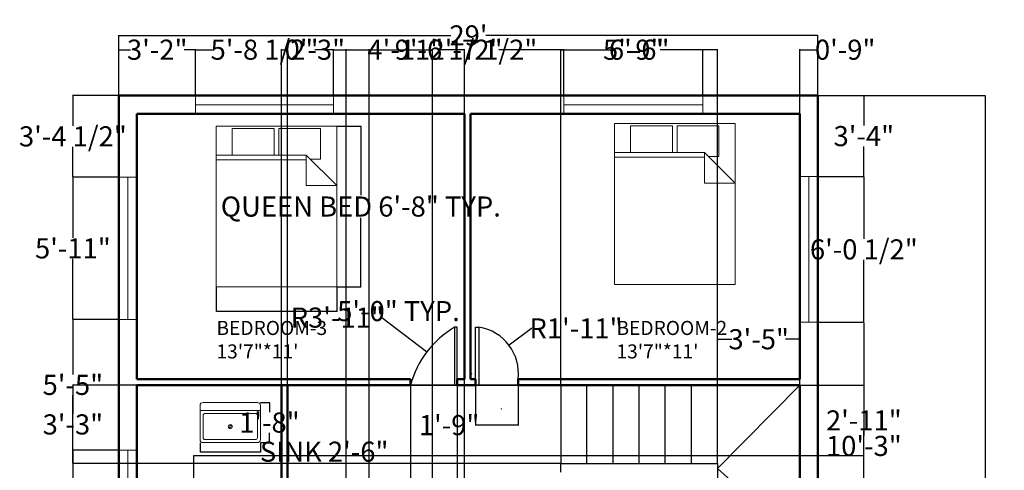
# Model space of a CAD drawing. Units: inches. Extents: x 430 to 924, y 262 to 758.
# Tile 3 of 3: x 434 to 924, y 534 to 758. Entities that reach past the tile are written whole.
import ezdxf

# ---------------------------------------------------------------- set-up
doc = ezdxf.new("R2010")
doc.units = ezdxf.units.IN
doc.header["$MEASUREMENT"] = 0
for name, color, linetype, lineweight in [('A-ANNO-DIMS', 2, 'Continuous', 18), ('A-AREA-IDEN', 7, 'Continuous', 25), ('A-DOOR', 4, 'Continuous', 25), ('A-FLOR-CASE', 9, 'Continuous', 25), ('A-FLOR-FIXT', 9, 'Continuous', 18), ('A-FLOR-STRS', 7, 'Continuous', 25), ('A-FURN', 9, 'Continuous', 18), ('A-GLAZ', 3, 'Continuous', 18), ('A-WALL', 7, 'Continuous', 50)]:
    doc.layers.add(name, color=color, linetype=linetype, lineweight=lineweight)
doc.styles.get("Standard").update_dxf_attribs({"font": 'arial.ttf'})
doc.dimstyles.get("Standard").update_dxf_attribs({"dimtxt": 10, "dimasz": 0.18, "dimexe": 0.18, "dimexo": 0.0625, "dimgap": 0.09, "dimtad": 0, "dimtih": 1, "dimtoh": 1, "dimdec": 0, "dimzin": 0, "dimdsep": 46, "dimlunit": 3, "dimtxsty": 'Standard', "dimcen": 0.09, "dimadec": 0, "dimazin": 0, "dimtfac": 1, "dimtdec": 0, "dimtofl": 0, "dimtmove": 0, "dimatfit": 3, "dimfxl": 1, "dimtolj": 1, "dimtzin": 0, "dimarcsym": 0})

# ---------------------------------------------------------------- blocks, each defined once
blk = doc.blocks.new('Bed - Queen')
for p, q in [((0, -80.00003), (0, 0)), ((0, 0), (59.99999, 0)), ((59.99999, 0), (59.99999, -80.00003)), ((7.99999, -1.2), (28.79998, -1.2)), ((7.99999, -14.4), (7.99999, -1.2)), ((28.79998, -1.2), (28.79998, -14.4)), ((31.19999, -1.2), (51.99999, -1.2)), ((31.19999, -14.4), (31.19999, -1.2)), ((51.99999, -1.2), (51.99999, -16.4)), ((0, -14.4), (44.8, -14.4)), ((59.99999, -29.6), (44.8, -14.4)), ((44.8, -14.4), (44.8, -29.6)), ((44.8, -16.8), (0, -16.8)), ((51.99999, -16.4), (46.79936, -16.4)), ((44.8, -29.6), (59.99999, -29.6)), ((59.99999, -80.00003), (0, -80.00003))]:
    blk.add_line(p, q)
blk = doc.blocks.new('Sink-single - 30 in top')
blk.add_line((-15, -3.999996), (15, -3.999996))
for points in [[(-13.5, 0), (13.5, 0)], [(-15, -18.499996), (-15, -1.5)], [(15, -1.5), (15, -18.499996)], [(-13.5, -17.499996), (-13.5, -6.499996)], [(-12.5, -5.499996), (12.5, -5.499996)], [(13.5, -6.499996), (13.5, -17.499996)], [(12.5, -18.499996), (-12.5, -18.499996)], [(13.5, -19.999996), (-13.5, -19.999996)]]:
    blk.add_lwpolyline(points)
for radius in [1, 0.5]:
    blk.add_circle((0, -11.999996), radius)
for centre, radius, start, end in [((-13.5, -1.5), 1.5, 90, 180), ((13.5, -1.5), 1.5, 0, 90), ((-12.5, -6.499996), 1, 90, 180), ((12.5, -6.499996), 1, 0, 90), ((-13.5, -18.499996), 1.5, 180, 270), ((-12.5, -17.499996), 1, 180, 270), ((12.5, -17.499996), 1, 270, 0), ((13.5, -18.499996), 1.5, 270, 0)]:
    blk.add_arc(centre, radius, start, end)
blk = doc.blocks.new('*D5')
at = {"layer": 'A-ANNO-DIMS', "color": 0, "lineweight": -2, "transparency": 16777216}
for p, q in [((483.32, 720.12), (483.32, 750.18)), ((483.5, 750), (648.65, 750)), ((831.14, 750), (665.98, 750)), ((831.32, 720.12), (831.32, 750.18))]:
    blk.add_line(p, q, dxfattribs=at)
at = {"layer": 'A-ANNO-DIMS', "color": 0, "transparency": 16777216}
for points in [[(483.5, 750.03), (483.5, 749.97), (483.32, 750)], [(831.14, 750.03), (831.14, 749.97), (831.32, 750)]]:
    blk.add_solid(points, dxfattribs=at)
at = {"layer": 'Defpoints', "color": 0, "transparency": 16777216}
for p in [(831.32, 750), (483.32, 720.05), (831.32, 720.05)]:
    blk.add_point(p, dxfattribs=at)
at = {"layer": 'A-ANNO-DIMS', "color": 0, "transparency": 16777216, "insert": (657.32, 750), "char_height": 10, "attachment_point": 5}
blk.add_mtext("\\A1;29'", dxfattribs=at)
blk = doc.blocks.new('*D6')
at = {"layer": 'A-ANNO-DIMS', "color": 0, "lineweight": -2, "transparency": 16777216}
for p, q in [((831.38, 720.05), (914.81, 720.05)), ((914.63, 719.87), (914.63, 515.25)), ((914.63, 300.23), (914.63, 504.86)), ((831.38, 300.05), (914.81, 300.05))]:
    blk.add_line(p, q, dxfattribs=at)
at = {"layer": 'A-ANNO-DIMS', "color": 0, "transparency": 16777216}
for points in [[(914.6, 719.87), (914.66, 719.87), (914.63, 720.05)], [(914.6, 300.23), (914.66, 300.23), (914.63, 300.05)]]:
    blk.add_solid(points, dxfattribs=at)
at = {"layer": 'Defpoints', "color": 0, "transparency": 16777216}
for p in [(831.32, 720.05), (831.32, 300.05), (914.63, 300.05)]:
    blk.add_point(p, dxfattribs=at)
at = {"layer": 'A-ANNO-DIMS', "color": 0, "transparency": 16777216, "insert": (914.63, 510.05), "char_height": 10, "attachment_point": 5}
blk.add_mtext("\\A1;35'", dxfattribs=at)
blk = doc.blocks.new('*D7')
at = {"layer": 'A-ANNO-DIMS', "color": 0, "lineweight": -2, "transparency": 16777216}
for p, q in [((591.83, 704.91), (603.95, 704.91)), ((603.77, 704.73), (603.77, 670.48)), ((603.77, 625.09), (603.77, 659.35)), ((591.83, 624.91), (603.95, 624.91))]:
    blk.add_line(p, q, dxfattribs=at)
at = {"layer": 'A-ANNO-DIMS', "color": 0, "transparency": 16777216}
for points in [[(603.74, 704.73), (603.8, 704.73), (603.77, 704.91)], [(603.74, 625.09), (603.8, 625.09), (603.77, 624.91)]]:
    blk.add_solid(points, dxfattribs=at)
at = {"layer": 'Defpoints', "color": 0, "transparency": 16777216}
for p in [(591.77, 704.91), (603.77, 704.91), (591.77, 624.91)]:
    blk.add_point(p, dxfattribs=at)
at = {"layer": 'A-ANNO-DIMS', "color": 0, "transparency": 16777216, "insert": (603.77, 664.91), "char_height": 10, "attachment_point": 5}
blk.add_mtext('\\A1;QUEEN BED 6\'-8" TYP.', dxfattribs=at)
blk = doc.blocks.new('*D8')
at = {"layer": 'A-ANNO-DIMS', "color": 0, "lineweight": -2, "transparency": 16777216}
for p, q in [((531.77, 624.85), (531.77, 612.73)), ((591.77, 624.85), (591.77, 612.73)), ((531.95, 612.91), (591.59, 612.91)), ((591.77, 612.91), (591.95, 612.91))]:
    blk.add_line(p, q, dxfattribs=at)
at = {"layer": 'A-ANNO-DIMS', "color": 0, "transparency": 16777216}
for points in [[(531.95, 612.94), (531.95, 612.88), (531.77, 612.91)], [(591.59, 612.94), (591.59, 612.88), (591.77, 612.91)]]:
    blk.add_solid(points, dxfattribs=at)
at = {"layer": 'Defpoints', "color": 0, "transparency": 16777216}
for p in [(531.77, 624.91), (591.77, 624.91), (591.77, 612.91)]:
    blk.add_point(p, dxfattribs=at)
at = {"layer": 'A-ANNO-DIMS', "color": 0, "transparency": 16777216, "insert": (622.52, 612.91), "char_height": 10, "attachment_point": 5}
blk.add_mtext('\\A1;5\'-0" TYP.', dxfattribs=at)
blk = doc.blocks.new('*D11')
at = {"layer": 'A-ANNO-DIMS', "color": 0, "lineweight": -2, "transparency": 16777216}
for p, q in [((523.75, 547.42), (523.75, 542.8)), ((553.75, 547.42), (553.75, 542.8)), ((523.93, 542.98), (553.57, 542.98)), ((553.75, 542.98), (553.93, 542.98))]:
    blk.add_line(p, q, dxfattribs=at)
at = {"layer": 'A-ANNO-DIMS', "color": 0, "transparency": 16777216}
for points in [[(523.93, 543.01), (523.93, 542.95), (523.75, 542.98)], [(553.57, 543.01), (553.57, 542.95), (553.75, 542.98)]]:
    blk.add_solid(points, dxfattribs=at)
at = {"layer": 'Defpoints', "color": 0, "transparency": 16777216}
for p in [(523.75, 547.48), (553.75, 547.48), (553.75, 542.98)]:
    blk.add_point(p, dxfattribs=at)
at = {"layer": 'A-ANNO-DIMS', "color": 0, "transparency": 16777216, "insert": (585.53, 542.98), "char_height": 10, "attachment_point": 5}
blk.add_mtext('\\A1;SINK 2\'-6"', dxfattribs=at)
blk = doc.blocks.new('*D12')
at = {"layer": 'A-ANNO-DIMS', "color": 0, "lineweight": -2, "transparency": 16777216}
for p, q in [((553.82, 567.48), (558.43, 567.48)), ((558.25, 567.3), (558.25, 562.68)), ((558.25, 547.66), (558.25, 552.29)), ((553.82, 547.48), (558.43, 547.48))]:
    blk.add_line(p, q, dxfattribs=at)
at = {"layer": 'A-ANNO-DIMS', "color": 0, "transparency": 16777216}
for points in [[(558.22, 567.3), (558.28, 567.3), (558.25, 567.48)], [(558.22, 547.66), (558.28, 547.66), (558.25, 547.48)]]:
    blk.add_solid(points, dxfattribs=at)
at = {"layer": 'Defpoints', "color": 0, "transparency": 16777216}
for p in [(553.75, 567.48), (558.25, 567.48), (553.75, 547.48)]:
    blk.add_point(p, dxfattribs=at)
at = {"layer": 'A-ANNO-DIMS', "color": 0, "transparency": 16777216, "insert": (558.25, 557.48), "char_height": 10, "attachment_point": 5}
blk.add_mtext('\\A1;1\'-8"', dxfattribs=at)
blk = doc.blocks.new('*D15')
at = {"layer": 'A-ANNO-DIMS', "color": 0, "lineweight": -2, "transparency": 16777216}
for p, q in [((483.32, 720.12), (483.32, 743.09)), ((483.5, 742.91), (489.04, 742.91)), ((521.35, 742.91), (515.8, 742.91)), ((521.53, 720.12), (521.53, 743.09))]:
    blk.add_line(p, q, dxfattribs=at)
at = {"layer": 'A-ANNO-DIMS', "color": 0, "transparency": 16777216}
for points in [[(483.5, 742.94), (483.5, 742.88), (483.32, 742.91)], [(521.35, 742.94), (521.35, 742.88), (521.53, 742.91)]]:
    blk.add_solid(points, dxfattribs=at)
at = {"layer": 'Defpoints', "color": 0, "transparency": 16777216}
for p in [(521.53, 742.91), (483.32, 720.05), (521.53, 720.05)]:
    blk.add_point(p, dxfattribs=at)
at = {"layer": 'A-ANNO-DIMS', "color": 0, "transparency": 16777216, "insert": (502.42, 742.91), "char_height": 10, "attachment_point": 5}
blk.add_mtext('\\A1;3\'-2"', dxfattribs=at)
blk = doc.blocks.new('*D16')
at = {"layer": 'A-ANNO-DIMS', "color": 0, "lineweight": -2, "transparency": 16777216}
for p, q in [((521.53, 720.12), (521.53, 743.09)), ((521.71, 742.91), (530.79, 742.91)), ((589.94, 742.91), (580.86, 742.91)), ((590.12, 720.12), (590.12, 743.09))]:
    blk.add_line(p, q, dxfattribs=at)
at = {"layer": 'A-ANNO-DIMS', "color": 0, "transparency": 16777216}
for points in [[(521.71, 742.94), (521.71, 742.88), (521.53, 742.91)], [(589.94, 742.94), (589.94, 742.88), (590.12, 742.91)]]:
    blk.add_solid(points, dxfattribs=at)
at = {"layer": 'Defpoints', "color": 0, "transparency": 16777216}
for p in [(590.12, 742.91), (521.53, 720.05), (590.12, 720.05)]:
    blk.add_point(p, dxfattribs=at)
at = {"layer": 'A-ANNO-DIMS', "color": 0, "transparency": 16777216, "insert": (555.83, 742.91), "char_height": 10, "attachment_point": 5}
blk.add_mtext('\\A1;5\'-8 1/2"', dxfattribs=at)
blk = doc.blocks.new('*D17')
at = {"layer": 'A-ANNO-DIMS', "color": 0, "lineweight": -2, "transparency": 16777216}
for p, q in [((590.12, 720.12), (590.12, 743.09)), ((590.3, 742.91), (622.43, 742.91)), ((704.63, 742.91), (672.5, 742.91)), ((704.81, 720.12), (704.81, 743.09))]:
    blk.add_line(p, q, dxfattribs=at)
at = {"layer": 'A-ANNO-DIMS', "color": 0, "transparency": 16777216}
for points in [[(590.3, 742.94), (590.3, 742.88), (590.12, 742.91)], [(704.63, 742.94), (704.63, 742.88), (704.81, 742.91)]]:
    blk.add_solid(points, dxfattribs=at)
at = {"layer": 'Defpoints', "color": 0, "transparency": 16777216}
for p in [(704.81, 742.91), (590.12, 720.05), (704.81, 720.05)]:
    blk.add_point(p, dxfattribs=at)
at = {"layer": 'A-ANNO-DIMS', "color": 0, "transparency": 16777216, "insert": (647.47, 742.91), "char_height": 10, "attachment_point": 5}
blk.add_mtext('\\A1;9\'-6 1/2"', dxfattribs=at)
blk = doc.blocks.new('*D18')
at = {"layer": 'A-ANNO-DIMS', "color": 0, "lineweight": -2, "transparency": 16777216}
for p, q in [((704.81, 720.12), (704.81, 743.09)), ((704.99, 742.91), (726, 742.91)), ((773.78, 742.91), (752.76, 742.91)), ((773.96, 720.12), (773.96, 743.09))]:
    blk.add_line(p, q, dxfattribs=at)
at = {"layer": 'A-ANNO-DIMS', "color": 0, "transparency": 16777216}
for points in [[(704.99, 742.94), (704.99, 742.88), (704.81, 742.91)], [(773.78, 742.94), (773.78, 742.88), (773.96, 742.91)]]:
    blk.add_solid(points, dxfattribs=at)
at = {"layer": 'Defpoints', "color": 0, "transparency": 16777216}
for p in [(773.96, 742.91), (704.81, 720.05), (773.96, 720.05)]:
    blk.add_point(p, dxfattribs=at)
at = {"layer": 'A-ANNO-DIMS', "color": 0, "transparency": 16777216, "insert": (739.38, 742.91), "char_height": 10, "attachment_point": 5}
blk.add_mtext('\\A1;5\'-9"', dxfattribs=at)
blk = doc.blocks.new('*D19')
at = {"layer": 'A-ANNO-DIMS', "color": 0, "lineweight": -2, "transparency": 16777216}
for p, q in [((831.38, 720.05), (854.35, 720.05)), ((854.17, 719.87), (854.17, 705.14)), ((854.17, 680.01), (854.17, 694.75)), ((831.38, 679.83), (854.35, 679.83))]:
    blk.add_line(p, q, dxfattribs=at)
at = {"layer": 'A-ANNO-DIMS', "color": 0, "transparency": 16777216}
for points in [[(854.14, 719.87), (854.2, 719.87), (854.17, 720.05)], [(854.14, 680.01), (854.2, 680.01), (854.17, 679.83)]]:
    blk.add_solid(points, dxfattribs=at)
at = {"layer": 'Defpoints', "color": 0, "transparency": 16777216}
for p in [(831.32, 720.05), (831.32, 679.83), (854.17, 679.83)]:
    blk.add_point(p, dxfattribs=at)
at = {"layer": 'A-ANNO-DIMS', "color": 0, "transparency": 16777216, "insert": (854.17, 699.94), "char_height": 10, "attachment_point": 5}
blk.add_mtext('\\A1;3\'-4"', dxfattribs=at)
blk = doc.blocks.new('*D20')
at = {"layer": 'A-ANNO-DIMS', "color": 0, "lineweight": -2, "transparency": 16777216}
for p, q in [((831.38, 679.83), (854.35, 679.83)), ((854.17, 679.65), (854.17, 648.84)), ((854.17, 607.5), (854.17, 638.32)), ((831.38, 607.32), (854.35, 607.32))]:
    blk.add_line(p, q, dxfattribs=at)
at = {"layer": 'A-ANNO-DIMS', "color": 0, "transparency": 16777216}
for points in [[(854.14, 679.65), (854.2, 679.65), (854.17, 679.83)], [(854.14, 607.5), (854.2, 607.5), (854.17, 607.32)]]:
    blk.add_solid(points, dxfattribs=at)
at = {"layer": 'Defpoints', "color": 0, "transparency": 16777216}
for p in [(831.32, 679.83), (831.32, 607.32), (854.17, 607.32)]:
    blk.add_point(p, dxfattribs=at)
at = {"layer": 'A-ANNO-DIMS', "color": 0, "transparency": 16777216, "insert": (854.17, 643.58), "char_height": 10, "attachment_point": 5}
blk.add_mtext('\\A1;6\'-0 1/2"', dxfattribs=at)
blk = doc.blocks.new('*D21')
at = {"layer": 'A-ANNO-DIMS', "color": 0, "lineweight": -2, "transparency": 16777216}
for p, q in [((831.38, 607.32), (854.35, 607.32)), ((854.17, 607.14), (854.17, 551.05)), ((854.17, 484.56), (854.17, 540.65)), ((831.38, 484.38), (854.35, 484.38))]:
    blk.add_line(p, q, dxfattribs=at)
at = {"layer": 'A-ANNO-DIMS', "color": 0, "transparency": 16777216}
for points in [[(854.14, 607.14), (854.2, 607.14), (854.17, 607.32)], [(854.14, 484.56), (854.2, 484.56), (854.17, 484.38)]]:
    blk.add_solid(points, dxfattribs=at)
at = {"layer": 'Defpoints', "color": 0, "transparency": 16777216}
for p in [(831.32, 607.32), (831.32, 484.38), (854.17, 484.38)]:
    blk.add_point(p, dxfattribs=at)
at = {"layer": 'A-ANNO-DIMS', "color": 0, "transparency": 16777216, "insert": (854.17, 545.85), "char_height": 10, "attachment_point": 5}
blk.add_mtext('\\A1;10\'-3"', dxfattribs=at)
blk = doc.blocks.new('*D25')
at = {"layer": 'A-ANNO-DIMS', "color": 0, "lineweight": -2, "transparency": 16777216}
for p, q in [((483.25, 720.05), (460.24, 720.05)), ((460.42, 719.87), (460.42, 705.08)), ((460.42, 679.75), (460.42, 694.55)), ((483.25, 679.57), (460.24, 679.57))]:
    blk.add_line(p, q, dxfattribs=at)
at = {"layer": 'A-ANNO-DIMS', "color": 0, "transparency": 16777216}
for points in [[(460.39, 719.87), (460.45, 719.87), (460.42, 720.05)], [(460.39, 679.75), (460.45, 679.75), (460.42, 679.57)]]:
    blk.add_solid(points, dxfattribs=at)
at = {"layer": 'Defpoints', "color": 0, "transparency": 16777216}
for p in [(483.32, 720.05), (460.42, 679.57), (483.32, 679.57)]:
    blk.add_point(p, dxfattribs=at)
at = {"layer": 'A-ANNO-DIMS', "color": 0, "transparency": 16777216, "insert": (460.42, 699.81), "char_height": 10, "attachment_point": 5}
blk.add_mtext('\\A1;3\'-4 1/2"', dxfattribs=at)
blk = doc.blocks.new('*D26')
at = {"layer": 'A-ANNO-DIMS', "color": 0, "lineweight": -2, "transparency": 16777216}
for p, q in [((483.25, 679.57), (460.24, 679.57)), ((460.42, 679.39), (460.42, 649.31)), ((460.42, 608.84), (460.42, 638.92)), ((483.25, 608.66), (460.24, 608.66))]:
    blk.add_line(p, q, dxfattribs=at)
at = {"layer": 'A-ANNO-DIMS', "color": 0, "transparency": 16777216}
for points in [[(460.39, 679.39), (460.45, 679.39), (460.42, 679.57)], [(460.39, 608.84), (460.45, 608.84), (460.42, 608.66)]]:
    blk.add_solid(points, dxfattribs=at)
at = {"layer": 'Defpoints', "color": 0, "transparency": 16777216}
for p in [(483.32, 679.57), (460.42, 608.66), (483.32, 608.66)]:
    blk.add_point(p, dxfattribs=at)
at = {"layer": 'A-ANNO-DIMS', "color": 0, "transparency": 16777216, "insert": (460.42, 644.11), "char_height": 10, "attachment_point": 5}
blk.add_mtext('\\A1;5\'-11"', dxfattribs=at)
blk = doc.blocks.new('*D27')
at = {"layer": 'A-ANNO-DIMS', "color": 0, "lineweight": -2, "transparency": 16777216}
for p, q in [((483.25, 608.66), (460.24, 608.66)), ((460.42, 608.48), (460.42, 581.39)), ((460.42, 543.96), (460.42, 571.04)), ((483.25, 543.78), (460.24, 543.78))]:
    blk.add_line(p, q, dxfattribs=at)
at = {"layer": 'A-ANNO-DIMS', "color": 0, "transparency": 16777216}
for points in [[(460.39, 608.48), (460.45, 608.48), (460.42, 608.66)], [(460.39, 543.96), (460.45, 543.96), (460.42, 543.78)]]:
    blk.add_solid(points, dxfattribs=at)
at = {"layer": 'Defpoints', "color": 0, "transparency": 16777216}
for p in [(483.32, 608.66), (460.42, 543.78), (483.32, 543.78)]:
    blk.add_point(p, dxfattribs=at)
at = {"layer": 'A-ANNO-DIMS', "color": 0, "transparency": 16777216, "insert": (460.42, 576.22), "char_height": 10, "attachment_point": 5}
blk.add_mtext('\\A1;5\'-5"', dxfattribs=at)
blk = doc.blocks.new('*D28')
at = {"layer": 'A-ANNO-DIMS', "color": 0, "lineweight": -2, "transparency": 16777216}
for p, q in [((483.25, 543.78), (460.24, 543.78)), ((460.42, 543.6), (460.42, 518.31)), ((460.42, 482.49), (460.42, 507.78)), ((483.25, 482.31), (460.24, 482.31))]:
    blk.add_line(p, q, dxfattribs=at)
at = {"layer": 'A-ANNO-DIMS', "color": 0, "transparency": 16777216}
for points in [[(460.39, 543.6), (460.45, 543.6), (460.42, 543.78)], [(460.39, 482.49), (460.45, 482.49), (460.42, 482.31)]]:
    blk.add_solid(points, dxfattribs=at)
at = {"layer": 'Defpoints', "color": 0, "transparency": 16777216}
for p in [(483.32, 543.78), (460.42, 482.31), (483.32, 482.31)]:
    blk.add_point(p, dxfattribs=at)
at = {"layer": 'A-ANNO-DIMS', "color": 0, "transparency": 16777216, "insert": (460.42, 513.05), "char_height": 10, "attachment_point": 5}
blk.add_mtext('\\A1;5\'-1 1/2"', dxfattribs=at)
blk = doc.blocks.new('*D35')
at = {"layer": 'A-ANNO-DIMS', "color": 0, "lineweight": -2, "transparency": 16777216}
for p, q in [((596.53, 380.21), (596.53, 743.09)), ((596.71, 742.91), (608.45, 742.91)), ((655.14, 742.91), (643.39, 742.91)), ((655.32, 380.21), (655.32, 743.09))]:
    blk.add_line(p, q, dxfattribs=at)
at = {"layer": 'A-ANNO-DIMS', "color": 0, "transparency": 16777216}
for points in [[(596.71, 742.94), (596.71, 742.88), (596.53, 742.91)], [(655.14, 742.94), (655.14, 742.88), (655.32, 742.91)]]:
    blk.add_solid(points, dxfattribs=at)
at = {"layer": 'Defpoints', "color": 0, "transparency": 16777216}
for p in [(655.32, 742.91), (596.53, 380.15), (655.32, 380.15)]:
    blk.add_point(p, dxfattribs=at)
at = {"layer": 'A-ANNO-DIMS', "color": 0, "transparency": 16777216, "insert": (625.92, 742.91), "char_height": 10, "attachment_point": 5}
blk.add_mtext('\\A1;4\'-11"', dxfattribs=at)
blk = doc.blocks.new('*D36')
at = {"layer": 'A-ANNO-DIMS', "color": 0, "lineweight": -2, "transparency": 16777216}
for p, q in [((703.32, 576.12), (703.32, 743.09)), ((703.5, 742.91), (728.92, 742.91)), ((781.17, 742.91), (755.74, 742.91)), ((781.35, 576.12), (781.35, 743.09))]:
    blk.add_line(p, q, dxfattribs=at)
at = {"layer": 'A-ANNO-DIMS', "color": 0, "transparency": 16777216}
for points in [[(703.5, 742.94), (703.5, 742.88), (703.32, 742.91)], [(781.17, 742.94), (781.17, 742.88), (781.35, 742.91)]]:
    blk.add_solid(points, dxfattribs=at)
at = {"layer": 'Defpoints', "color": 0, "transparency": 16777216}
for p in [(781.35, 742.91), (703.32, 576.05), (781.35, 576.05)]:
    blk.add_point(p, dxfattribs=at)
at = {"layer": 'A-ANNO-DIMS', "color": 0, "transparency": 16777216, "insert": (742.33, 742.91), "char_height": 10, "attachment_point": 5}
blk.add_mtext('\\A1;6\'-6"', dxfattribs=at)
blk = doc.blocks.new('*D37')
at = {"layer": 'A-ANNO-DIMS', "color": 0, "lineweight": -2, "transparency": 16777216}
for p, q in [((781.35, 576.12), (781.35, 599.09)), ((781.53, 598.91), (788.45, 598.91)), ((822.14, 598.91), (815.21, 598.91)), ((822.32, 576.12), (822.32, 599.09))]:
    blk.add_line(p, q, dxfattribs=at)
at = {"layer": 'A-ANNO-DIMS', "color": 0, "transparency": 16777216}
for points in [[(781.53, 598.94), (781.53, 598.88), (781.35, 598.91)], [(822.14, 598.94), (822.14, 598.88), (822.32, 598.91)]]:
    blk.add_solid(points, dxfattribs=at)
at = {"layer": 'Defpoints', "color": 0, "transparency": 16777216}
for p in [(822.32, 598.91), (781.35, 576.05), (822.32, 576.05)]:
    blk.add_point(p, dxfattribs=at)
at = {"layer": 'A-ANNO-DIMS', "color": 0, "transparency": 16777216, "insert": (801.83, 598.91), "char_height": 10, "attachment_point": 5}
blk.add_mtext('\\A1;3\'-5"', dxfattribs=at)
blk = doc.blocks.new('*D38')
at = {"layer": 'A-ANNO-DIMS', "color": 0, "lineweight": -2, "transparency": 16777216}
for p, q in [((703.25, 576.05), (460.24, 576.05)), ((460.42, 575.87), (460.42, 561.75)), ((460.42, 537.23), (460.42, 551.36)), ((703.25, 537.05), (460.24, 537.05))]:
    blk.add_line(p, q, dxfattribs=at)
at = {"layer": 'A-ANNO-DIMS', "color": 0, "transparency": 16777216}
for points in [[(460.39, 575.87), (460.45, 575.87), (460.42, 576.05)], [(460.39, 537.23), (460.45, 537.23), (460.42, 537.05)]]:
    blk.add_solid(points, dxfattribs=at)
at = {"layer": 'Defpoints', "color": 0, "transparency": 16777216}
for p in [(703.32, 576.05), (460.42, 537.05), (703.32, 537.05)]:
    blk.add_point(p, dxfattribs=at)
at = {"layer": 'A-ANNO-DIMS', "color": 0, "transparency": 16777216, "insert": (460.42, 556.55), "char_height": 10, "attachment_point": 5}
blk.add_mtext('\\A1;3\'-3"', dxfattribs=at)
blk = doc.blocks.new('*D41')
at = {"layer": 'A-ANNO-DIMS', "color": 0, "lineweight": -2, "transparency": 16777216}
for p, q in [((822.32, 484.44), (822.32, 743.09)), ((822.5, 742.91), (831.14, 742.91)), ((831.32, 484.44), (831.32, 743.09)), ((831.32, 742.91), (831.5, 742.91))]:
    blk.add_line(p, q, dxfattribs=at)
at = {"layer": 'A-ANNO-DIMS', "color": 0, "transparency": 16777216}
for points in [[(822.5, 742.94), (822.5, 742.88), (822.32, 742.91)], [(831.14, 742.94), (831.14, 742.88), (831.32, 742.91)]]:
    blk.add_solid(points, dxfattribs=at)
at = {"layer": 'Defpoints', "color": 0, "transparency": 16777216}
for p in [(831.32, 742.91), (822.32, 484.38), (831.32, 484.38)]:
    blk.add_point(p, dxfattribs=at)
at = {"layer": 'A-ANNO-DIMS', "color": 0, "transparency": 16777216, "insert": (844.88, 742.91), "char_height": 10, "attachment_point": 5}
blk.add_mtext('\\A1;0\'-9"', dxfattribs=at)
blk = doc.blocks.new('*D43')
at = {"layer": 'A-ANNO-DIMS', "color": 0, "lineweight": -2, "transparency": 16777216}
for p, q in [((564.38, 576.05), (854.35, 576.05)), ((854.17, 575.87), (854.17, 563.64)), ((854.17, 541.19), (854.17, 553.42)), ((564.38, 541.01), (854.35, 541.01))]:
    blk.add_line(p, q, dxfattribs=at)
at = {"layer": 'A-ANNO-DIMS', "color": 0, "transparency": 16777216}
for points in [[(854.14, 575.87), (854.2, 575.87), (854.17, 576.05)], [(854.14, 541.19), (854.2, 541.19), (854.17, 541.01)]]:
    blk.add_solid(points, dxfattribs=at)
at = {"layer": 'Defpoints', "color": 0, "transparency": 16777216}
for p in [(564.32, 576.05), (854.17, 576.05), (564.32, 541.01)]:
    blk.add_point(p, dxfattribs=at)
at = {"layer": 'A-ANNO-DIMS', "color": 0, "transparency": 16777216, "insert": (854.17, 558.53), "char_height": 10, "attachment_point": 5}
blk.add_mtext('\\A1;2\'-11"', dxfattribs=at)
blk = doc.blocks.new('*D45')
at = {"layer": 'A-ANNO-DIMS', "color": 0, "lineweight": -2, "transparency": 16777216}
for p, q in [((564.32, 576.12), (564.32, 743.09)), ((564.5, 742.91), (567.14, 742.91)), ((567.32, 576.12), (567.32, 743.09)), ((567.32, 742.91), (567.5, 742.91))]:
    blk.add_line(p, q, dxfattribs=at)
at = {"layer": 'A-ANNO-DIMS', "color": 0, "transparency": 16777216}
for points in [[(564.5, 742.94), (564.5, 742.88), (564.32, 742.91)], [(567.14, 742.94), (567.14, 742.88), (567.32, 742.91)]]:
    blk.add_solid(points, dxfattribs=at)
at = {"layer": 'Defpoints', "color": 0, "transparency": 16777216}
for p in [(567.32, 742.91), (564.32, 576.05), (567.32, 576.05)]:
    blk.add_point(p, dxfattribs=at)
at = {"layer": 'A-ANNO-DIMS', "color": 0, "transparency": 16777216, "insert": (580.88, 742.91), "char_height": 10, "attachment_point": 5}
blk.add_mtext('\\A1;0\'-3"', dxfattribs=at)
blk = doc.blocks.new('*D46')
at = {"layer": 'A-ANNO-DIMS', "color": 0, "lineweight": -2, "transparency": 16777216}
for p, q in [((628.55, 575.99), (628.55, 277.02)), ((651.7, 575.99), (651.7, 277.02)), ((628.73, 277.2), (651.52, 277.2)), ((651.7, 277.2), (651.88, 277.2))]:
    blk.add_line(p, q, dxfattribs=at)
at = {"layer": 'A-ANNO-DIMS', "color": 0, "transparency": 16777216}
for points in [[(628.73, 277.23), (628.73, 277.17), (628.55, 277.2)], [(651.52, 277.23), (651.52, 277.17), (651.7, 277.2)]]:
    blk.add_solid(points, dxfattribs=at)
at = {"layer": 'Defpoints', "color": 0, "transparency": 16777216}
for p in [(628.55, 576.05), (651.7, 576.05), (651.7, 277.2)]:
    blk.add_point(p, dxfattribs=at)
at = {"layer": 'A-ANNO-DIMS', "color": 0, "transparency": 16777216, "insert": (668.68, 277.2), "char_height": 10, "attachment_point": 5}
blk.add_mtext('\\A1;1\'-11"', dxfattribs=at)
blk = doc.blocks.new('*D47')
at = {"layer": 'A-ANNO-DIMS', "color": 0, "lineweight": -2, "transparency": 16777216}
for p, q in [((660.82, 578.99), (660.82, 556.02)), ((682.01, 578.99), (682.01, 556.02)), ((660.82, 556.2), (660.64, 556.2)), ((681.83, 556.2), (661, 556.2))]:
    blk.add_line(p, q, dxfattribs=at)
at = {"layer": 'A-ANNO-DIMS', "color": 0, "transparency": 16777216}
for points in [[(661, 556.23), (661, 556.17), (660.82, 556.2)], [(681.83, 556.23), (681.83, 556.17), (682.01, 556.2)]]:
    blk.add_solid(points, dxfattribs=at)
at = {"layer": 'Defpoints', "color": 0, "transparency": 16777216}
for p in [(660.82, 579.05), (682.01, 579.05), (660.82, 556.2)]:
    blk.add_point(p, dxfattribs=at)
at = {"layer": 'A-ANNO-DIMS', "color": 0, "transparency": 16777216, "insert": (647.73, 556.2), "char_height": 10, "attachment_point": 5}
blk.add_mtext('\\A1;1\'-9"', dxfattribs=at)
blk = doc.blocks.new('*D48')
at = {"layer": 'A-ANNO-DIMS', "color": 0, "lineweight": -2, "transparency": 16777216}
for p, q in [((607.88, 405.12), (607.88, 743.09)), ((608.06, 742.91), (639.32, 742.91)), ((639.5, 405.12), (639.5, 743.09)), ((639.5, 742.91), (639.68, 742.91))]:
    blk.add_line(p, q, dxfattribs=at)
at = {"layer": 'A-ANNO-DIMS', "color": 0, "transparency": 16777216}
for points in [[(608.06, 742.94), (608.06, 742.88), (607.88, 742.91)], [(639.32, 742.94), (639.32, 742.88), (639.5, 742.91)]]:
    blk.add_solid(points, dxfattribs=at)
at = {"layer": 'Defpoints', "color": 0, "transparency": 16777216}
for p in [(639.5, 742.91), (607.88, 405.05), (639.5, 405.05)]:
    blk.add_point(p, dxfattribs=at)
at = {"layer": 'A-ANNO-DIMS', "color": 0, "transparency": 16777216, "insert": (664.79, 742.91), "char_height": 10, "attachment_point": 5}
blk.add_mtext('\\A1;2\'-7 1/2"', dxfattribs=at)
blk = doc.blocks.new('*D52')
at = {"layer": 'A-ANNO-DIMS', "color": 0, "lineweight": -2, "transparency": 16777216}
for p, q in [((614.09, 609.68), (614.27, 609.68)), ((614.27, 609.68), (636.47, 592.79)), ((673.76, 564.35), (673.94, 564.35)), ((673.85, 564.26), (673.85, 564.44))]:
    blk.add_line(p, q, dxfattribs=at)
at = {"layer": 'A-ANNO-DIMS', "color": 0, "transparency": 16777216}
blk.add_solid([(636.49, 592.81), (636.45, 592.77), (636.61, 592.68)], dxfattribs=at)
at = {"layer": 'Defpoints', "color": 0, "transparency": 16777216}
for p in [(636.61, 592.68), (673.85, 564.35)]:
    blk.add_point(p, dxfattribs=at)
at = {"layer": 'A-ANNO-DIMS', "color": 0, "transparency": 16777216, "insert": (592.04, 609.68), "char_height": 10, "attachment_point": 5}
blk.add_mtext('\\A1;R3\'-11"', dxfattribs=at)
blk = doc.blocks.new('*D53')
at = {"layer": 'A-ANNO-DIMS', "color": 0, "lineweight": -2, "transparency": 16777216}
for p, q in [((688.65, 604.3), (677.66, 596.02)), ((688.83, 604.3), (688.65, 604.3)), ((658.87, 581.93), (659.05, 581.93)), ((658.96, 581.84), (658.96, 582.02))]:
    blk.add_line(p, q, dxfattribs=at)
at = {"layer": 'A-ANNO-DIMS', "color": 0, "transparency": 16777216}
blk.add_solid([(677.64, 596.04), (677.68, 596), (677.52, 595.91)], dxfattribs=at)
at = {"layer": 'Defpoints', "color": 0, "transparency": 16777216}
for p in [(677.52, 595.91), (658.96, 581.93)]:
    blk.add_point(p, dxfattribs=at)
at = {"layer": 'A-ANNO-DIMS', "color": 0, "transparency": 16777216, "insert": (710.89, 604.3), "char_height": 10, "attachment_point": 5}
blk.add_mtext('\\A1;R1\'-11"', dxfattribs=at)

msp = doc.modelspace()

# ---------------------------------------------------------------- linework, layer by layer
at = {"layer": 'A-DOOR'}
for p, q in [((651.7, 604.89), (650.48, 604.89)), ((650.48, 604.89), (650.48, 576.05)), ((651.7, 579.05), (651.7, 604.89)), ((660.82, 579.05), (660.82, 604.89)), ((660.82, 604.89), (662.56, 604.89)), ((662.56, 604.89), (662.56, 576.05)), ((628.55, 576.05), (648.07, 576.05)), ((651.7, 576.05), (648.07, 576.05)), ((660.82, 576.05), (663.66, 576.05)), ((682.01, 576.05), (663.66, 576.05))]:
    msp.add_line(p, q, dxfattribs=at)
for centre, radius, start, end in [((673.85, 564.35), 46.79, 119.9685, 165.5188), ((658.96, 581.93), 23.24, 352.8813, 81.0788)]:
    msp.add_arc(centre, radius, start, end, dxfattribs=at)
at = {"layer": 'A-FLOR-CASE'}
for p, q in [((520.6, 456.05), (520.6, 541.01)), ((520.6, 541.01), (564.32, 541.01))]:
    msp.add_line(p, q, dxfattribs=at)
at = {"layer": 'A-FLOR-STRS'}
for p, q in [((703.32, 576.05), (703.32, 537.05)), ((716.35, 537.05), (716.35, 576.05)), ((729.35, 537.05), (729.35, 576.05)), ((742.35, 537.05), (742.35, 576.05)), ((755.35, 537.05), (755.35, 576.05)), ((768.35, 537.05), (768.35, 576.05)), ((781.35, 537.05), (781.35, 576.05)), ((781.35, 534.67), (822.32, 576.05)), ((703.32, 537.05), (781.16, 537.05)), ((703.32, 532.81), (703.32, 537.05)), ((781.35, 537.05), (781.16, 537.05)), ((781.35, 537.05), (781.35, 498.05)), ((781.35, 534.67), (822.32, 498.05))]:
    msp.add_line(p, q, dxfattribs=at)
at = {"layer": 'A-GLAZ'}
for p, q in [((521.53, 720.05), (521.53, 711.05)), ((590.12, 720.05), (590.12, 711.05)), ((704.81, 711.05), (704.81, 720.05)), ((773.96, 720.05), (773.96, 711.05)), ((521.53, 715.55), (590.12, 715.55)), ((704.81, 715.55), (773.96, 715.55)), ((483.32, 679.57), (492.32, 679.57)), ((487.82, 679.57), (487.82, 608.66)), ((822.32, 679.83), (831.32, 679.83)), ((826.82, 679.83), (826.82, 607.32)), ((483.32, 608.66), (492.32, 608.66)), ((822.32, 607.32), (831.32, 607.32)), ((483.32, 543.78), (492.32, 543.78)), ((487.82, 543.78), (487.82, 482.31))]:
    msp.add_line(p, q, dxfattribs=at)
at = {"layer": 'A-WALL'}
for p, q in [((492.32, 711.05), (655.32, 711.05)), ((492.32, 579.05), (492.32, 711.05)), ((655.32, 579.05), (655.32, 711.05)), ((658.32, 579.05), (658.32, 711.05)), ((658.32, 711.05), (822.32, 711.05)), ((822.32, 711.05), (822.32, 579.05)), ((492.32, 579.05), (628.55, 579.05)), ((628.55, 579.05), (628.55, 576.05)), ((651.7, 579.05), (651.7, 576.05)), ((651.7, 579.05), (655.32, 579.05)), ((658.32, 579.05), (660.82, 579.05)), ((660.82, 579.05), (660.82, 576.05)), ((682.01, 579.05), (682.01, 576.05)), ((682.01, 579.05), (822.32, 579.05)), ((492.32, 402.05), (492.32, 576.05)), ((492.32, 576.05), (628.55, 576.05)), ((564.32, 498.05), (564.32, 576.05)), ((567.32, 498.05), (567.32, 576.05)), ((651.7, 576.05), (660.82, 576.05)), ((682.01, 576.05), (822.32, 576.05)), ((822.32, 576.05), (822.32, 498.05))]:
    msp.add_line(p, q, dxfattribs=at)
msp.add_lwpolyline([(831.32, 720.05), (831.32, 300.05), (483.32, 300.05), (483.32, 720.05)], close=True, dxfattribs=at)

# ---------------------------------------------------------------- block references
at = {"layer": 'A-FLOR-FIXT'}
msp.add_blockref('Sink-single - 30 in top', (538.75, 567.48), dxfattribs=at)
at = {"layer": 'A-FURN'}
for p in [(730.06, 706.18), (531.77, 704.91)]:
    msp.add_blockref('Bed - Queen', p, dxfattribs=at)

# ---------------------------------------------------------------- texts
at = {"layer": 'A-AREA-IDEN', "char_height": 7, "attachment_point": 1}
for s, insert in [('BEDROOM-3\\P13\'7"*11\'', (531.91, 608.02)), ('BEDROOM-2\\P13\'7"*11\'', (731.04, 608.02))]:
    msp.add_mtext_dynamic_manual_height_columns(s, width=58.4467, gutter_width=1, heights=[0], dxfattribs=dict(at, insert=insert))

# ---------------------------------------------------------------- dimensions: what is measured, and where the dimension line sits
at = {"layer": 'A-ANNO-DIMS'}
for base, p1, p2, override, picture, middle in [((831.32, 750), (483.32, 720.05), (831.32, 720.05), {"dimclrd": 0, "dimclre": 0, "dimclrt": 0}, '*D5', (657.32, 750)), ((590.12, 742.91), (521.53, 720.05), (590.12, 720.05), {"dimdec": 1, "dimlfac": 1, "dimrnd": 0, "dimzin": 1, "dimdsep": 46, "dimlunit": 4, "dimfrac": 2}, '*D16', (555.83, 742.91)), ((704.81, 742.91), (590.12, 720.05), (704.81, 720.05), {"dimdec": 1, "dimlfac": 1, "dimrnd": 0, "dimzin": 1, "dimdsep": 46, "dimlunit": 4, "dimfrac": 2}, '*D17', (647.47, 742.91)), ((639.5, 742.91), (607.88, 405.05), (639.5, 405.05), {"dimdec": 1, "dimlfac": 1, "dimrnd": 0, "dimzin": 1, "dimdsep": 46, "dimlunit": 4, "dimfrac": 2}, '*D48', (664.79, 742.91)), ((521.53, 742.91), (483.32, 720.05), (521.53, 720.05), {"dimdec": 1, "dimlfac": 1, "dimrnd": 0, "dimzin": 1, "dimdsep": 46, "dimlunit": 4, "dimfrac": 2}, '*D15', (502.42, 742.91)), ((567.32, 742.91), (564.32, 576.05), (567.32, 576.05), {"dimdec": 1, "dimlfac": 1, "dimrnd": 0, "dimzin": 1, "dimdsep": 46, "dimlunit": 4, "dimfrac": 2}, '*D45', (580.88, 742.91)), ((655.32, 742.91), (596.53, 380.15), (655.32, 380.15), {"dimdec": 1, "dimlfac": 1, "dimrnd": 0, "dimzin": 1, "dimdsep": 46, "dimlunit": 4, "dimfrac": 2}, '*D35', (625.92, 742.91)), ((781.35, 742.91), (703.32, 576.05), (781.35, 576.05), {"dimdec": 1, "dimlfac": 1, "dimrnd": 0, "dimzin": 1, "dimdsep": 46, "dimlunit": 4, "dimfrac": 2}, '*D36', (742.33, 742.91)), ((773.9551, 742.9092), (704.8084, 720.0542), (773.9551, 720.0542), {"dimdec": 1, "dimlfac": 1, "dimrnd": 0, "dimzin": 1, "dimdsep": 46, "dimlunit": 4, "dimfrac": 2}, '*D18', (739.3817, 742.9092)), ((831.32, 742.91), (822.32, 484.38), (831.32, 484.38), {"dimdec": 1, "dimlfac": 1, "dimrnd": 0, "dimzin": 1, "dimdsep": 46, "dimlunit": 4, "dimfrac": 2}, '*D41', (844.88, 742.91)), ((822.32, 598.91), (781.35, 576.05), (822.32, 576.05), {"dimdec": 1, "dimlfac": 1, "dimrnd": 0, "dimzin": 1, "dimdsep": 46, "dimlunit": 4, "dimfrac": 2}, '*D37', (801.83, 598.91)), ((651.7007, 277.1992), (628.5501, 576.0542), (651.7007, 576.0542), {"dimdec": 1, "dimlfac": 1, "dimrnd": 0, "dimzin": 1, "dimdsep": 46, "dimlunit": 4, "dimfrac": 2}, '*D46', (668.6761, 277.1992))]:
    dim = msp.add_linear_dim(base=base, p1=p1, p2=p2, dimstyle='Standard', override=override, dxfattribs=at)
    dim.commit()
    dim.dimension.update_dxf_attribs({"geometry": picture, "text_midpoint": middle})
for base, p1, p2, angle, override, picture, middle in [((460.42, 679.57), (483.32, 720.05), (483.32, 679.57), 90, {"dimdec": 1, "dimlfac": 1, "dimrnd": 0, "dimzin": 1, "dimdsep": 46, "dimlunit": 4, "dimfrac": 2}, '*D25', (460.42, 699.81)), ((914.63, 300.05), (831.32, 720.05), (831.32, 300.05), 90, {"dimclrd": 0, "dimclre": 0, "dimclrt": 0}, '*D6', (914.63, 510.05)), ((854.17, 679.83), (831.32, 720.05), (831.32, 679.83), 90, {"dimdec": 1, "dimlfac": 1, "dimrnd": 0, "dimzin": 1, "dimdsep": 46, "dimlunit": 4, "dimfrac": 2}, '*D19', (854.17, 699.94)), ((460.42, 608.66), (483.32, 679.57), (483.32, 608.66), 90, {"dimdec": 1, "dimlfac": 1, "dimrnd": 0, "dimzin": 1, "dimdsep": 46, "dimlunit": 4, "dimfrac": 2}, '*D26', (460.42, 644.11)), ((854.17, 607.32), (831.32, 679.83), (831.32, 607.32), 90, {"dimdec": 1, "dimlfac": 1, "dimrnd": 0, "dimzin": 1, "dimdsep": 46, "dimlunit": 4, "dimfrac": 2}, '*D20', (854.17, 643.58)), ((460.42, 543.78), (483.32, 608.66), (483.32, 543.78), 90, {"dimdec": 1, "dimlfac": 1, "dimrnd": 0, "dimzin": 1, "dimdsep": 46, "dimlunit": 4, "dimfrac": 2}, '*D27', (460.42, 576.22)), ((854.17, 484.38), (831.32, 607.32), (831.32, 484.38), 90, {"dimdec": 1, "dimlfac": 1, "dimrnd": 0, "dimzin": 1, "dimdsep": 46, "dimlunit": 4, "dimfrac": 2}, '*D21', (854.17, 545.85)), ((660.82, 556.2), (682.01, 579.05), (660.82, 579.05), 180, {"dimdec": 1, "dimlfac": 1, "dimrnd": 0, "dimzin": 1, "dimdsep": 46, "dimlunit": 4, "dimfrac": 2}, '*D47', (647.73, 556.2)), ((460.42, 537.05), (703.32, 576.05), (703.32, 537.05), 90, {"dimdec": 1, "dimlfac": 1, "dimrnd": 0, "dimzin": 1, "dimdsep": 46, "dimlunit": 4, "dimfrac": 2}, '*D38', (460.42, 556.55)), ((854.17, 576.05), (564.32, 541.01), (564.32, 576.05), 90, {"dimdec": 1, "dimlfac": 1, "dimrnd": 0, "dimzin": 1, "dimdsep": 46, "dimlunit": 4, "dimfrac": 2}, '*D43', (854.17, 558.53)), ((558.25, 567.48), (553.75, 547.48), (553.75, 567.48), 90, {"dimdec": 1, "dimlfac": 1, "dimrnd": 0, "dimzin": 1, "dimdsep": 46, "dimlunit": 4, "dimfrac": 2}, '*D12', (558.25, 557.48)), ((460.42, 482.31), (483.32, 543.78), (483.32, 482.31), 90, {"dimdec": 1, "dimlfac": 1, "dimrnd": 0, "dimzin": 1, "dimdsep": 46, "dimlunit": 4, "dimfrac": 2}, '*D28', (460.42, 513.05))]:
    dim = msp.add_linear_dim(base=base, p1=p1, p2=p2, angle=angle, dimstyle='Standard', override=override, dxfattribs=at)
    dim.commit()
    dim.dimension.update_dxf_attribs({"geometry": picture, "text_midpoint": middle})
dim = msp.add_linear_dim(base=(603.77, 704.91), p1=(591.77, 624.91), p2=(591.77, 704.91), angle=90, text='QUEEN BED <> TYP.', dimstyle='Standard', override={"dimdec": 1, "dimlfac": 1, "dimrnd": 0, "dimzin": 1, "dimdsep": 46, "dimlunit": 4, "dimfrac": 2}, dxfattribs=at)
dim.commit()
dim.dimension.update_dxf_attribs({"geometry": '*D7', "text_midpoint": (603.77, 664.91)})
for base, p1, p2, text, picture, middle in [((591.77, 612.91), (531.77, 624.91), (591.77, 624.91), '<> TYP.', '*D8', (622.52, 612.91)), ((553.75, 542.98), (523.75, 547.48), (553.75, 547.48), 'SINK <>', '*D11', (585.53, 542.98))]:
    dim = msp.add_linear_dim(base=base, p1=p1, p2=p2, text=text, dimstyle='Standard', override={"dimdec": 1, "dimlfac": 1, "dimrnd": 0, "dimzin": 1, "dimdsep": 46, "dimlunit": 4, "dimfrac": 2}, dxfattribs=at)
    dim.commit()
    dim.dimension.update_dxf_attribs({"geometry": picture, "text_midpoint": middle})
for center, mpoint, picture, middle in [((673.85, 564.35), (636.61, 592.68), '*D52', (592.04, 609.68)), ((658.96, 581.93), (677.52, 595.91), '*D53', (710.89, 604.3))]:
    dim = msp.add_radius_dim(center=center, mpoint=mpoint, dimstyle='Standard', override={"dimdec": 1, "dimlfac": 1, "dimrnd": 0, "dimzin": 1, "dimdsep": 46, "dimlunit": 4, "dimfrac": 2}, dxfattribs=at)
    dim.commit()
    dim.dimension.update_dxf_attribs({"geometry": picture, "text_midpoint": middle, "dimtype": 164})

doc.saveas('drawing.dxf')
